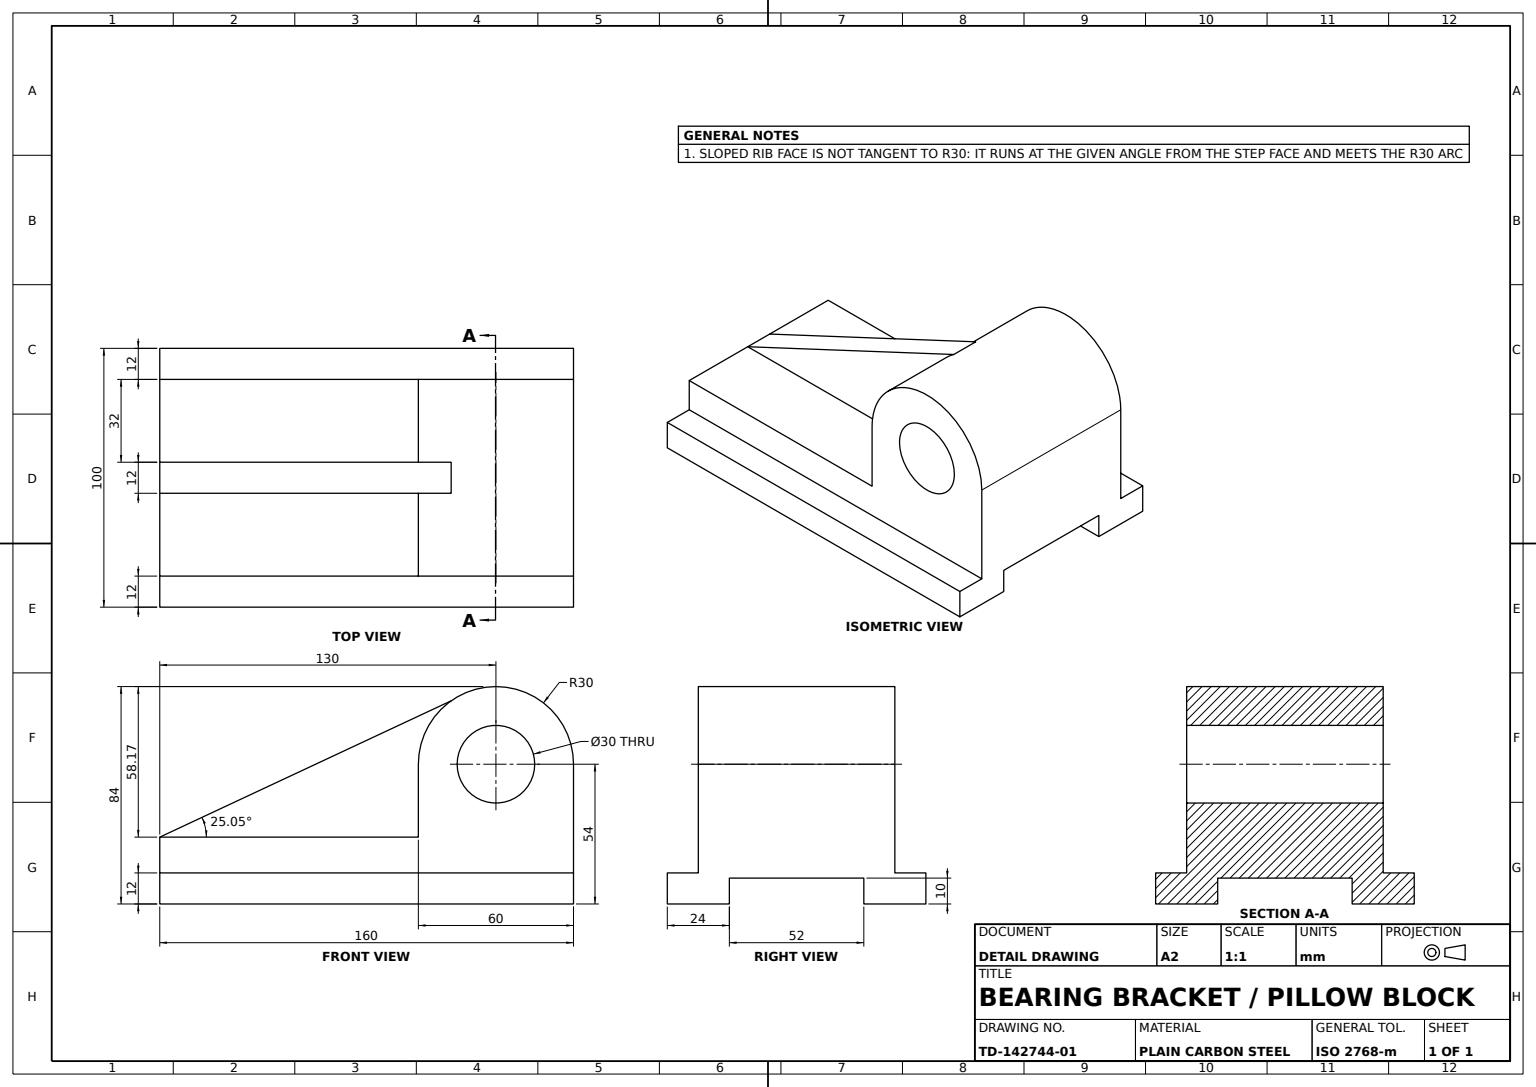
SolidWorks part; units mm, degrees
material "Plain Carbon Steel"
ref_plane "Front Plane" through (0, 0, 0) normal (0, 0, 1) x (1, 0, 0)
ref_plane "Top Plane" through (0, 0, 0) normal (0, 1, 0) x (1, 0, 0)
ref_plane "Right Plane" through (0, 0, 0) normal (1, 0, 0) x (0, 0, -1)
sketch "Base Slide Profile Sketch" plane through (0, 0, 0) normal (0, 0, 1) x (1, 0, 0)
  line L0 (-26, 0) -> (26, 0)
  line L1 (-26, 0) -> (-26, -10)
  line L2 (-26, -10) -> (-50, -10)
  line L3 (-50, -10) -> (-50, 2)
  line L4 (-50, 2) -> (-38, 2)
  line L5 (-38, 2) -> (-38, 74)
  line L6 (-38, 74) -> (38, 74)
  line L8 (26, 0) -> (26, -10)
  line L9 (38, 2) -> (38, 74)
  line L10 (50, 2) -> (38, 2)
  line L11 (50, -10) -> (50, 2)
  line L12 (26, -10) -> (50, -10)
  line L13 (-38, 2) -> (-38, 14)
  line L14 (-38, 14) -> (38, 14)
  line L15 (38, 14) -> (38, 2)
  point P4 (0, 0)
  dimension "D1" = 52
  dimension "D2" = 10
  dimension "D3" = 12
  dimension "D4" = 12
  dimension "D5" = 24
  dimension "D6" = 84
  dimension "D7" = 12
extrude "Base Block 160" add sketch "Base Slide Profile Sketch" along normal blind 160 contours L14 L5 L4 L3 L2 L1 L0 L8 L12 L11 L10 L9 | L5 L14 L9 L6
sketch "Bearing Block Outline Sketch" plane through (38, 0, 0) normal (1, 0, 0) x (0, 0, -1)
  line L0 (0, -10) -> (0, 44)
  line L2 (-160, 2) -> (-160, 15.8289)
  line L3 (-160, 2) -> (-160, 74) construction
  line L5 (-60, 44) -> (-60, 15.8289)
  line L6 (-60, 2) -> (0, 2)
  line L7 (0, 44) -> (0, 2)
  line L8 (-160, 15.8289) -> (-60, 15.8289)
  line L9 (-160, 15.8289) -> (-160, 74)
  line L10 (-160, 74) -> (0, 74)
  line L11 (0, 74) -> (0, 44)
  line L13 (-160, 74) -> (0, 74) construction
  arc A0 (0, 44) -> (-60, 44) centre (-30, 44) ccw
  circle A1 centre (-30, 44) radius 15
  line M6 (0, 2) -> (0, 74)
  line M7 (0, 74) -> (-160, 74)
  line M8 (-160, 74) -> (-160, 2)
  dimension "D3" = 30
  dimension "D1" = 54
  dimension "D2" = 60
  dimension "D4" = 30
  dimension "D5" = 58.1711
extrude "Bearing Block Shaping Cut" cut sketch "Bearing Block Outline Sketch" against normal through all contours A0 L10 L8 L5 M8 | A0 M6 M7
sketch "Support Rib Sketch" plane through (0, 0, 0) normal (1, 0, 0) x (0, 0, -1)
  line L0 (-160, 15.8289) -> (-47.3116, 68.5012)
  line L1 (-160, 15.8289) -> (-60, 15.8289)
  line L2 (-60, 15.8289) -> (-60, 44)
  arc A0 (0, 44) -> (-60, 44) centre (-30, 44) ccw construction
  arc A1 (-60, 44) -> (-47.3116, 68.5012) centre (-30, 44) cw
  dimension "D1" = 12.6884
extrude "Support Rib 12" add sketch "Support Rib Sketch" along normal mid plane 12
sketch "Bore Sketch" plane through (38, 0, 0) normal (1, 0, 0) x (0, 0, -1)
  circle A0 centre (-30, 44) radius 15
  dimension "D3" = 30
  dimension "D1" = 54
  dimension "D2" = 30
extrude "Bore Ø30" cut sketch "Bore Sketch" against normal through all
